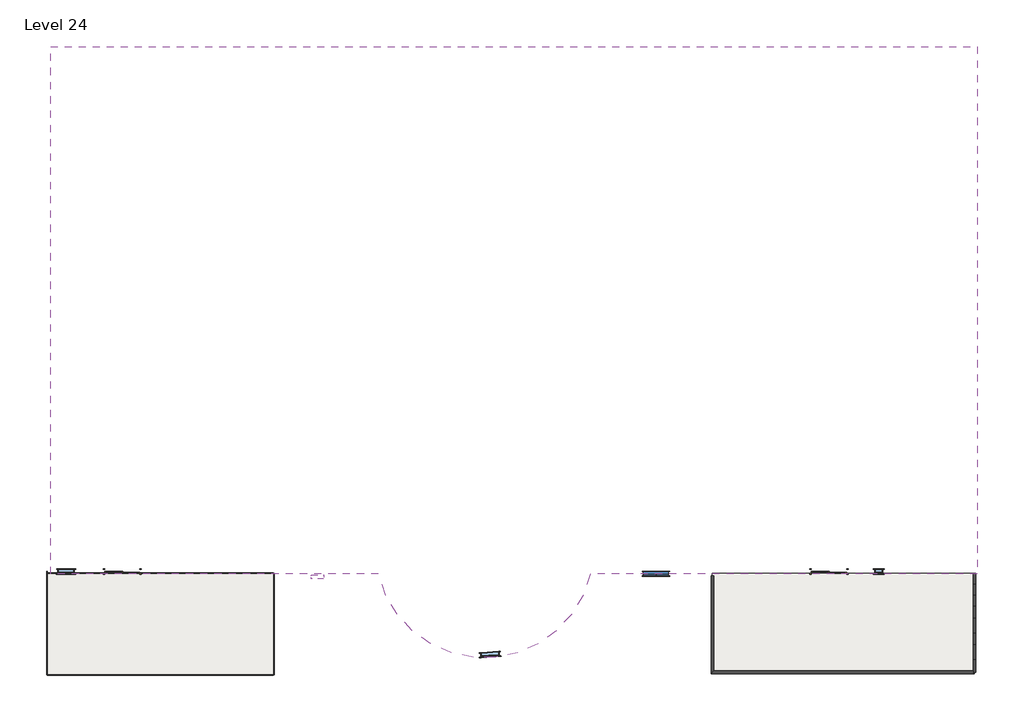
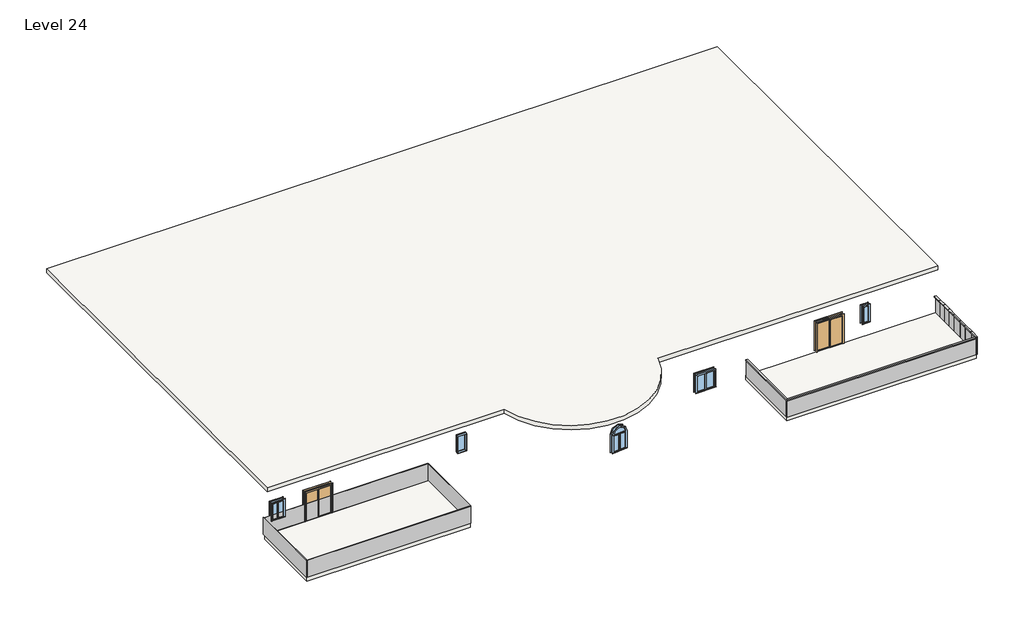
# One storey: 14 plates, 11 members, 5 windows, 3 slabs, 2 doors.
"""IFC4 building model written with IfcOpenShell, lengths in millimetres."""

from ifc_helpers import new_model, si_unit, point, frame, frame_2d, origin, place, context, project, spatial, polyline, circle_curve, trimmed, segment, composite_curve, outline, extrude, transform, mapped, element, save
from components import door_076b30e0, member_75074519, member_47bfaf8a, member_ae70dd35, member_41daa855, member_b9da2caa, member_623bfa76, member_d7af48b5, member_0d72fb60, system_panel_glazed_7af1c9c3, system_panel_glazed_a854efd3, system_panel_glazed_e5e35a93, system_panel_glazed_70ce58d2, system_panel_glazed_b1e6bfa8, system_panel_glazed_da164243, system_panel_glazed_d9f0472a, system_panel_glazed_b96adab1, system_panel_glazed_773201f3, system_panel_glazed_8ecd3908, window_cf4adaea, window_a765b88f, window_bb17773d, window_0862ab64, window_80bd9af0

model = new_model("IFC4")

# Units and contexts
model_context = context("Model", 3, world=origin())
ifc_project = project(units=[si_unit("LENGTHUNIT", "METRE", prefix="MILLI")], contexts=[model_context])

# Site, building, storey
site = spatial("IfcSite", under=ifc_project)
building = spatial("IfcBuilding", under=site)
storey = spatial("IfcBuildingStorey", under=building, Name="Level 24", Elevation=39928.8)

# Doors
placement = place(None, origin())
door_shape = door_076b30e0(model_context)
element("IfcDoor", 1, ObjectType="Door-Double-Sliding : 68\" x 80\"", at=placement, inside=storey, context=model_context, shape_type="MappedRepresentation", body=[
    mapped(door_shape, transform((-16166.185279, -12227.7237084, 39928.8), x_axis=(-1.0, 0.0, 0.0), y_axis=(0.0, -1.0, 0.0), z_axis=(0.0, 0.0, 1.0))),
])
element("IfcDoor", 2, ObjectType="Door-Double-Sliding : 68\" x 80\"", at=placement, inside=storey, context=model_context, shape_type="MappedRepresentation", body=[
    mapped(door_shape, transform((18377.814721, -12227.7237084, 39928.8), x_axis=(-1.0, 0.0, 0.0), y_axis=(0.0, -1.0, 0.0), z_axis=(0.0, 0.0, 1.0))),
])

# Members
member_shape = member_75074519(model_context)
element("IfcMember", 3, ObjectType="Rectangular Mullion : 2.5\" x 5\" rectangular", at=placement, inside=storey, context=model_context, shape_type="MappedRepresentation", body=[
    mapped(member_shape, transform((25489.814721, -17286.7294032, 41148.0), x_axis=(1.0, 0.0, 0.0), y_axis=(0.0, 1.0, 0.0), z_axis=(0.0, 0.0, 1.0))),
])
member_2_shape = member_47bfaf8a(model_context)
element("IfcMember", 4, ObjectType="Rectangular Mullion : 2.5\" x 5\" rectangular", at=placement, inside=storey, context=model_context, shape_type="MappedRepresentation", body=[
    mapped(member_2_shape, transform((25489.814721, -14645.1294032, 41148.0), x_axis=(0.0, 0.0, 1.0), y_axis=(-1.0, 0.0, 0.0), z_axis=(0.0, -1.0, 0.0))),
])
member_3_shape = member_ae70dd35(model_context)
element("IfcMember", 5, ObjectType="Rectangular Mullion : 2.5\" x 5\" rectangular", at=placement, inside=storey, context=model_context, shape_type="MappedRepresentation", body=[
    mapped(member_3_shape, transform((25489.814721, -15356.3294032, 41148.0), x_axis=(0.0, 0.0, 1.0), y_axis=(-1.0, 0.0, 0.0), z_axis=(0.0, -1.0, 0.0))),
])
element("IfcMember", 6, ObjectType="Rectangular Mullion : 2.5\" x 5\" rectangular", at=placement, inside=storey, context=model_context, shape_type="MappedRepresentation", body=[
    mapped(member_2_shape, transform((25489.814721, -17286.7294032, 41148.0), x_axis=(0.0, 0.0, 1.0), y_axis=(-1.0, 0.0, 0.0), z_axis=(0.0, -1.0, 0.0))),
])
member_4_shape = member_41daa855(model_context)
element("IfcMember", 7, ObjectType="Rectangular Mullion : 2.5\" x 5\" rectangular", at=placement, inside=storey, context=model_context, shape_type="MappedRepresentation", body=[
    mapped(member_4_shape, transform((12687.3363499, -12564.9789867, 41148.0), x_axis=(0.0, 0.0, 1.0), y_axis=(1.0, 0.0, 0.0), z_axis=(0.0, 1.0, 0.0))),
])
member_5_shape = member_b9da2caa(model_context)
element("IfcMember", 8, ObjectType="Rectangular Mullion : 2.5\" x 5\" rectangular", at=placement, inside=storey, context=model_context, shape_type="MappedRepresentation", body=[
    mapped(member_5_shape, transform((25489.814721, -12982.7256066, 41148.0), x_axis=(0.0, 0.0, 1.0), y_axis=(-1.0, 0.0, 0.0), z_axis=(0.0, -1.0, 0.0))),
])
element("IfcMember", 9, ObjectType="Rectangular Mullion : 2.5\" x 5\" rectangular", at=placement, inside=storey, context=model_context, shape_type="MappedRepresentation", body=[
    mapped(member_5_shape, transform((25489.814721, -13509.1275049, 41148.0), x_axis=(0.0, 0.0, 1.0), y_axis=(-1.0, 0.0, 0.0), z_axis=(0.0, -1.0, 0.0))),
])
element("IfcMember", 10, ObjectType="Rectangular Mullion : 2.5\" x 5\" rectangular", at=placement, inside=storey, context=model_context, shape_type="MappedRepresentation", body=[
    mapped(member_5_shape, transform((25489.814721, -14035.5294032, 41148.0), x_axis=(0.0, 0.0, 1.0), y_axis=(-1.0, 0.0, 0.0), z_axis=(0.0, -1.0, 0.0))),
])
member_6_shape = member_623bfa76(model_context)
element("IfcMember", 11, ObjectType="Rectangular Mullion : 2.5\" x 5\" rectangular", at=placement, inside=storey, context=model_context, shape_type="MappedRepresentation", body=[
    mapped(member_6_shape, transform((25489.814721, -15940.5294032, 41148.0), x_axis=(0.0, 0.0, 1.0), y_axis=(-1.0, 0.0, 0.0), z_axis=(0.0, -1.0, 0.0))),
])
member_7_shape = member_d7af48b5(model_context)
element("IfcMember", 12, ObjectType="Rectangular Mullion : 2.5\" x 5\" rectangular", at=placement, inside=storey, context=model_context, shape_type="MappedRepresentation", body=[
    mapped(member_7_shape, transform((25489.814721, -16677.1294032, 41148.0), x_axis=(0.0, 0.0, 1.0), y_axis=(-1.0, 0.0, 0.0), z_axis=(0.0, -1.0, 0.0))),
])
member_8_shape = member_0d72fb60(model_context)
element("IfcMember", 13, ObjectType="Rectangular Mullion : 2.5\" x 5\" rectangular", at=placement, inside=storey, context=model_context, shape_type="MappedRepresentation", body=[
    mapped(member_8_shape, transform((12687.3363499, -17286.7294032, 41148.0), x_axis=(0.0, 0.0, 1.0), y_axis=(0.0, 1.0, 0.0), z_axis=(-1.0, 0.0, 0.0))),
])

# Plates
system_panel_glazed_shape = system_panel_glazed_7af1c9c3(model_context)
element("IfcPlate", 14, ObjectType="System Panel : Glazed", at=placement, inside=storey, context=model_context, shape_type="MappedRepresentation", body=[
    mapped(system_panel_glazed_shape, transform((25489.814721, -16981.9294032, 39928.8), x_axis=(0.0, -1.0, 0.0), y_axis=(1.0, 0.0, 0.0), z_axis=(0.0, 0.0, 1.0))),
])
element("IfcPlate", 15, ObjectType="System Panel : Glazed", at=placement, inside=storey, context=model_context, shape_type="MappedRepresentation", body=[
    mapped(system_panel_glazed_shape, transform((25489.814721, -14340.3294032, 39928.8), x_axis=(0.0, -1.0, 0.0), y_axis=(1.0, 0.0, 0.0), z_axis=(0.0, 0.0, 1.0))),
])
system_panel_glazed_2_shape = system_panel_glazed_a854efd3(model_context)
element("IfcPlate", 16, ObjectType="System Panel : Glazed", at=placement, inside=storey, context=model_context, shape_type="MappedRepresentation", body=[
    mapped(system_panel_glazed_2_shape, transform((25489.814721, -15000.7294032, 39928.8), x_axis=(0.0, -1.0, 0.0), y_axis=(1.0, 0.0, 0.0), z_axis=(0.0, 0.0, 1.0))),
])
system_panel_glazed_3_shape = system_panel_glazed_e5e35a93(model_context)
element("IfcPlate", 17, ObjectType="System Panel : Glazed", at=placement, inside=storey, context=model_context, shape_type="MappedRepresentation", body=[
    mapped(system_panel_glazed_3_shape, transform((12687.3363499, -14925.8541949, 39928.8), x_axis=(0.0, 1.0, 0.0), y_axis=(-1.0, 0.0, 0.0), z_axis=(0.0, 0.0, 1.0))),
])
system_panel_glazed_4_shape = system_panel_glazed_70ce58d2(model_context)
element("IfcPlate", 18, ObjectType="System Panel : Glazed", at=placement, inside=storey, context=model_context, shape_type="MappedRepresentation", body=[
    mapped(system_panel_glazed_4_shape, transform((25489.814721, -12719.5246575, 39928.8), x_axis=(0.0, -1.0, 0.0), y_axis=(1.0, 0.0, 0.0), z_axis=(0.0, 0.0, 1.0))),
])
element("IfcPlate", 19, ObjectType="System Panel : Glazed", at=placement, inside=storey, context=model_context, shape_type="MappedRepresentation", body=[
    mapped(system_panel_glazed_4_shape, transform((25489.814721, -13772.3284541, 39928.8), x_axis=(0.0, -1.0, 0.0), y_axis=(1.0, 0.0, 0.0), z_axis=(0.0, 0.0, 1.0))),
])
element("IfcPlate", 20, ObjectType="System Panel : Glazed", at=placement, inside=storey, context=model_context, shape_type="MappedRepresentation", body=[
    mapped(system_panel_glazed_4_shape, transform((25489.814721, -13245.9265558, 39928.8), x_axis=(0.0, -1.0, 0.0), y_axis=(1.0, 0.0, 0.0), z_axis=(0.0, 0.0, 1.0))),
])
system_panel_glazed_5_shape = system_panel_glazed_b1e6bfa8(model_context)
element("IfcPlate", 21, ObjectType="System Panel : Glazed", at=placement, inside=storey, context=model_context, shape_type="MappedRepresentation", body=[
    mapped(system_panel_glazed_5_shape, transform((25489.814721, -16308.8294032, 39928.8), x_axis=(0.0, -1.0, 0.0), y_axis=(1.0, 0.0, 0.0), z_axis=(0.0, 0.0, 1.0))),
])
system_panel_glazed_6_shape = system_panel_glazed_da164243(model_context)
element("IfcPlate", 22, ObjectType="System Panel : Glazed", at=placement, inside=storey, context=model_context, shape_type="MappedRepresentation", body=[
    mapped(system_panel_glazed_6_shape, transform((25489.814721, -15648.4294032, 39928.8), x_axis=(0.0, -1.0, 0.0), y_axis=(1.0, 0.0, 0.0), z_axis=(0.0, 0.0, 1.0))),
])
system_panel_glazed_7_shape = system_panel_glazed_d9f0472a(model_context)
element("IfcPlate", 23, ObjectType="System Panel : Glazed", at=placement, inside=storey, context=model_context, shape_type="MappedRepresentation", body=[
    mapped(system_panel_glazed_7_shape, transform((19056.8255355, -17286.7294032, 39928.8), x_axis=(-1.0, 0.0, 0.0), y_axis=(0.0, -1.0, 0.0), z_axis=(0.0, 0.0, 1.0))),
])
system_panel_glazed_8_shape = system_panel_glazed_b96adab1(model_context)
element("IfcPlate", 24, ObjectType="System Panel : Glazed", at=placement, inside=storey, context=model_context, shape_type="MappedRepresentation", body=[
    mapped(system_panel_glazed_8_shape, transform((-14302.7926538, -12456.3237084, 39928.8), x_axis=(1.0, 0.0, 0.0), y_axis=(0.0, 1.0, 0.0), z_axis=(0.0, 0.0, 1.0))),
])
element("IfcPlate", 25, ObjectType="System Panel : Glazed", at=placement, inside=storey, context=model_context, shape_type="MappedRepresentation", body=[
    mapped(system_panel_glazed_8_shape, transform((-14302.7926538, -17395.7250056, 39928.8), x_axis=(-1.0, 0.0, 0.0), y_axis=(0.0, -1.0, 0.0), z_axis=(0.0, 0.0, 1.0))),
])
system_panel_glazed_9_shape = system_panel_glazed_773201f3(model_context)
element("IfcPlate", 26, ObjectType="System Panel : Glazed", at=placement, inside=storey, context=model_context, shape_type="MappedRepresentation", body=[
    mapped(system_panel_glazed_9_shape, transform((-8781.8000285, -14926.024357, 39928.8), x_axis=(0.0, -1.0, 0.0), y_axis=(1.0, 0.0, 0.0), z_axis=(0.0, 0.0, 1.0))),
])
system_panel_glazed_10_shape = system_panel_glazed_8ecd3908(model_context)
element("IfcPlate", 27, ObjectType="System Panel : Glazed", at=placement, inside=storey, context=model_context, shape_type="MappedRepresentation", body=[
    mapped(system_panel_glazed_10_shape, transform((-19823.785279, -14875.224357, 39928.8), x_axis=(0.0, 1.0, 0.0), y_axis=(-1.0, 0.0, 0.0), z_axis=(0.0, 0.0, 1.0))),
])

# Slabs
element("IfcSlab", 28, ObjectType="Generic - 12\"", at=placement, inside=storey, context=model_context, shape_type="SweptSolid", body=[
    extrude(outline(composite_curve([segment(polyline([(25642.214721, 13328.8447861), (25642.214721, -12477.5552139), (6723.9594464, -12477.5552139)]), True, "CONTINUOUS"), segment(trimmed(circle_curve(frame_2d((1537.614721, -11246.9221727)), 5330.3498284), [point((6723.9594464, -12477.5552139))], [point((-3648.7300045, -12477.5552139))], False, "CARTESIAN"), True, "CONTINUOUS"), segment(polyline([(-3648.7300045, -12477.5552139), (-19671.385279, -12477.5552139), (-19671.385279, 13328.8447861), (25642.214721, 13328.8447861)]), True, "CONTINUOUS")], self_intersect=False)), frame((0.0, 0.0, 42963.6098476), z_axis=(0.0, 0.0, 1.0), x_axis=(1.0, 0.0, 0.0)), (0.0, 0.0, 1.0), 304.8),
])
element("IfcSlab", 29, ObjectType="Generic - 12\"", at=placement, inside=storey, context=model_context, shape_type="SweptSolid", body=[
    extrude(outline(polyline([(25489.814721, -12433.2368115), (25489.814721, -17267.6794032), (12687.3363499, -17267.6794032), (12687.3363499, -12433.2368115), (25489.814721, -12433.2368115)])), frame((0.0, 0.0, 39624.0), z_axis=(0.0, 0.0, 1.0), x_axis=(1.0, 0.0, 0.0)), (0.0, 0.0, 1.0), 304.8),
])
element("IfcSlab", 30, ObjectType="Generic - 12\"", at=placement, inside=storey, context=model_context, shape_type="SweptSolid", body=[
    extrude(outline(polyline([(-8781.8000285, -12456.3237084), (-8781.8000285, -17395.7250056), (-19823.785279, -17395.7250056), (-19823.785279, -12456.3237084), (-8781.8000285, -12456.3237084)])), frame((0.0, 0.0, 39624.0), z_axis=(0.0, 0.0, 1.0), x_axis=(1.0, 0.0, 0.0)), (0.0, 0.0, 1.0), 304.8),
])

# Windows
window_shape = window_cf4adaea(model_context)
element("IfcWindow", 31, ObjectType="36\" x 48\"", at=placement, inside=storey, context=model_context, shape_type="MappedRepresentation", body=[
    mapped(window_shape, transform((1821.5964068, -16416.4921108, 39928.8), x_axis=(-0.996612399121061, -0.08224187448108751, 0.0), y_axis=(0.08224187448108751, -0.996612399121061, 0.0), z_axis=(0.0, 0.0, 1.0))),
])
window_2_shape = window_a765b88f(model_context)
element("IfcWindow", 32, ObjectType="Awning with Trim : 16\" x 48\"", at=placement, inside=storey, context=model_context, shape_type="MappedRepresentation", body=[
    mapped(window_2_shape, transform((20816.214721, -12354.7237084, 39928.8), x_axis=(-1.0, 0.0, 0.0), y_axis=(0.0, -1.0, 0.0), z_axis=(0.0, 0.0, 1.0))),
])
window_3_shape = window_bb17773d(model_context)
element("IfcWindow", 33, ObjectType="Casement Dbl with Trim : 32\" x 48\"", at=placement, inside=storey, context=model_context, shape_type="MappedRepresentation", body=[
    mapped(window_3_shape, transform((-18909.385279, -12335.6737084, 39853.6293246), x_axis=(-1.0, 0.0, 0.0), y_axis=(0.0, -1.0, 0.0), z_axis=(0.0, 0.0, 1.0))),
])
window_4_shape = window_0862ab64(model_context)
element("IfcWindow", 34, ObjectType="Casement Dbl with Trim : 48\" x 48\"", at=placement, inside=storey, context=model_context, shape_type="MappedRepresentation", body=[
    mapped(window_4_shape, transform((9924.3594464, -12437.2737084, 39022.1053459), x_axis=(-1.0, 0.0, 0.0), y_axis=(0.0, -1.0, 0.0), z_axis=(0.0, 0.0, 1.0))),
])
window_5_shape = window_80bd9af0(model_context)
element("IfcWindow", 35, ObjectType="Fixed : 24\" x 48\"", at=placement, inside=storey, context=model_context, shape_type="MappedRepresentation", body=[
    mapped(window_5_shape, transform((-6577.685279, -12617.2007309, 40463.3711489), x_axis=(1.0, 0.0, 0.0), y_axis=(0.0, 1.0, 0.0), z_axis=(0.0, 0.0, 1.0))),
])

save(model, "model.ifc")

# Revit data of these elements
# Type "Door-Double-Sliding : 68\" x 80\""
#   Type Mark = "10"
#   Construction Type Id = "opn-d45"
#   Assembly Code = "C1020"
#   Analytic Construction = "Wood frame, double glass door "
#   Thickness = 0' - 2"
#   Thermal Resistance (R) = 1.8150 (h·ft²·°F)/BTU
#   Heat Transfer Coefficient (U) = 0.5510 BTU/(h·ft²·°F)
#   Height = 6' - 8"
#   Rail Width = 0' - 2"
#   Stiles = 0' - 2"
#   Trim Projection Ext = 0' - 1"
#   Trim Projection Int = 0' - 1"
#   Trim Width = 0' - 3"
#   Width = 5' - 8"
#   Define Thermal Properties by = 1
#   Glazing = Glass
#   Panel Material = Wood - Birch - Solid Stained Light Low Gloss
#   Trim Material = Paint - Sienna
#   Visual Light Transmittance = 0
#   Solar Heat Gain Coefficient = 0
#   Function = (empty or 0)
#   Wall Closure = (empty or 0)
# Type "Rectangular Mullion : 2.5\" x 5\" rectangular"
#   built-in parameter 1007304 = 0.416667 (stored number, unit not read)
#   built-in parameter 1007301 = 0.104167 (stored number, unit not read)
#   built-in parameter 1007300 = 0.104167 (stored number, unit not read)
# Type "System Panel : Glazed"
#   Construction Type Id = "GSP4R"
#   Analytic Construction = "1/8 in Pilkington single glazing"
#   Visual Light Transmittance = 0.9
#   Solar Heat Gain Coefficient = 0.86
#   Heat Transfer Coefficient (U) = 1.18115 BTU/(h·ft²·°F)
# Type "Generic - 12\""
#   Assembly Code = "B1010"
#   Function = 0
#   Layers, outside or top first: 1' - 0" no material (function 1)
# Type "36\" x 48\""
#   Type Mark = "38"
#   Construction Type Id = "SGL"
#   Assembly Code = "B2020100"
#   Analytic Construction = "Large single-glazed windows"
#   Visual Light Transmittance = 0.9
#   Solar Heat Gain Coefficient = 0.86
#   Heat Transfer Coefficient (U) = 0.979472 BTU/(h·ft²·°F)
#   Height = 4' - 0"
#   Default Sill Height = 3' - 0"
#   Trim Projection - Ext. = 0' - 0 1/2"
#   Trim Projection - Int. = 0' - 0 3/4"
#   Trim Width - Exterior = 0' - 3 1/2"
#   Trim Width - Interior = 0' - 3 1/2"
#   Width = 3' - 0"
#   Window Inset = 0' - 0 3/4"
#   Define Thermal Properties by = 1
#   Glass Pane Material = Glass
#   Sash Material = Sash
#   Trim Exterior Material = Trim
#   Trim Interior Material = Trim
#   Wall Closure = (empty or 0)
# Type "Awning with Trim : 16\" x 48\""
#   Type Mark = "14"
#   Construction Type Id = "GSP4R"
#   Assembly Code = "B2020100"
#   Analytic Construction = "1/8 in Pilkington single glazing"
#   Visual Light Transmittance = 0.9
#   Solar Heat Gain Coefficient = 0.78
#   Heat Transfer Coefficient (U) = 0.6496 BTU/(h·ft²·°F)
#   Height = 4' - 0"
#   Default Sill Height = 3' - 0"
#   Trim Projection - Ext. = 0' - 0 1/2"
#   Trim Projection - Int. = 0' - 0 3/4"
#   Trim Width - Exterior = 0' - 3 1/2"
#   Trim Width - Interior = 0' - 3 1/2"
#   Width = 1' - 4"
#   Window Inset = 0' - 0 3/4"
#   Define Thermal Properties by = 1
#   Glass Pane Material = Glass
#   Sash Material = Sash
#   Trim Exterior Material = Trim
#   Trim Interior Material = Trim
#   Wall Closure = (empty or 0)
# Type "Casement Dbl with Trim : 32\" x 48\""
#   Type Mark = "36"
#   Construction Type Id = "GSP4R"
#   Assembly Code = "B2020100"
#   Analytic Construction = "1/8 in Pilkington single glazing"
#   Visual Light Transmittance = 0.9
#   Solar Heat Gain Coefficient = 0.78
#   Heat Transfer Coefficient (U) = 0.6496 BTU/(h·ft²·°F)
#   Height = 4' - 0"
#   Default Sill Height = 3' - 0"
#   Trim Projection - Ext. = 0' - 0 1/2"
#   Trim Projection - Int. = 0' - 0 3/4"
#   Trim Width - Exterior = 0' - 3 1/2"
#   Trim Width - Interior = 0' - 3 1/2"
#   Width = 2' - 8"
#   Window Inset = 0' - 0 3/4"
#   Define Thermal Properties by = 1
#   Glass Pane Material = Glass
#   Sash Material = Sash
#   Trim Exterior Material = Trim
#   Trim Interior Material = Trim
#   Wall Closure = (empty or 0)
# Type "Casement Dbl with Trim : 48\" x 48\""
#   Type Mark = "34"
#   Construction Type Id = "GSP4R"
#   Assembly Code = "B2020100"
#   Analytic Construction = "1/8 in Pilkington single glazing"
#   Visual Light Transmittance = 0.9
#   Solar Heat Gain Coefficient = 0.78
#   Heat Transfer Coefficient (U) = 0.6496 BTU/(h·ft²·°F)
#   Height = 4' - 0"
#   Default Sill Height = 3' - 0"
#   Trim Projection - Ext. = 0' - 0 1/2"
#   Trim Projection - Int. = 0' - 0 3/4"
#   Trim Width - Exterior = 0' - 3 1/2"
#   Trim Width - Interior = 0' - 3 1/2"
#   Width = 4' - 0"
#   Window Inset = 0' - 0 3/4"
#   Define Thermal Properties by = 1
#   Glass Pane Material = Glass
#   Sash Material = Sash
#   Trim Exterior Material = Trim
#   Trim Interior Material = Trim
#   Wall Closure = (empty or 0)
# Type "Fixed : 24\" x 48\""
#   Type Mark = "2"
#   Construction Type Id = "GSP4R"
#   Assembly Code = "B2020100"
#   Analytic Construction = "1/8 in Pilkington single glazing"
#   Visual Light Transmittance = 0.9
#   Solar Heat Gain Coefficient = 0.78
#   Heat Transfer Coefficient (U) = 0.6496 BTU/(h·ft²·°F)
#   Height = 4' - 0"
#   Default Sill Height = 3' - 0"
#   Width = 2' - 0"
#   Window Inset = 0' - 0 3/4"
#   Define Thermal Properties by = 1
#   Glass Pane Material = Glass
#   Sash Material = Sash
#   Wall Closure = (empty or 0)
# Elements 1, 2 (IfcDoor, "Door-Double-Sliding : 68\" x 80\"")
#   Phase Created = New Construction
#   Materials on its faces: "Paint - Sienna", "Wood - Birch - Solid Stained Light Low Gloss", "Glass"
# Elements 3, 4, 5, 6, 7, 8, 9, 10, 11, 12, 13 (IfcMember, "Rectangular Mullion : 2.5\" x 5\" rectangular")
#   Phase Created = New Construction
#   Materials on its faces: "Aluminum"
# Elements 14, 15, 16, 17, 18, 19, 20, 21, 22, 23, 24, 25, 26, 27 (IfcPlate, "System Panel : Glazed")
#   Phase Created = New Construction
#   Materials on its faces: "Glass"
# Element 28 (IfcSlab, "Generic - 12\"")
#   Height Offset From Level = 10' - 11.4807"
#   Phase Created = New Construction
#   Materials on its faces: "Default Floor"
# Elements 29, 30 (IfcSlab, "Generic - 12\"")
#   Height Offset From Level = 0' - 0"
#   Phase Created = New Construction
#   Materials on its faces: "Default Floor"
# Element 31 (IfcWindow, "36\" x 48\"")
#   Mark = "22"
#   Phase Created = New Construction
#   Materials on its faces: "Sash", "Trim", "Glass"
# Element 32 (IfcWindow, "Awning with Trim : 16\" x 48\"")
#   Mark = "56"
#   Phase Created = New Construction
#   Materials on its faces: "Sash", "Trim", "Glass"
# Element 33 (IfcWindow, "Casement Dbl with Trim : 32\" x 48\"")
#   Mark = "39"
#   Phase Created = New Construction
#   Materials on its faces: "Sash", "Trim", "Glass"
# Element 34 (IfcWindow, "Casement Dbl with Trim : 48\" x 48\"")
#   Mark = "5"
#   Phase Created = New Construction
#   Materials on its faces: "Sash", "Trim", "Glass"
# Element 35 (IfcWindow, "Fixed : 24\" x 48\"")
#   Mark = "73"
#   Phase Created = New Construction
#   Materials on its faces: "Sash", "Glass"
# Materials
#   "Glass": class "Glass", colour RGB 0 128 192, transparency 0.75, Description = "Soda Lime Glass", Cost = 0
#   "Wood - Birch - Solid Stained Light Low Gloss": class "Wood", colour RGB 210 159 95, transparency 0, Cost = 0
#   "Paint - Sienna": colour RGB 118 70 51, transparency 0, Cost = 0
#   "Sash": class "Wood", colour RGB 224 178 126, transparency 0
#   "Trim": class "Wood", colour RGB 224 178 126, transparency 0
#   "Aluminum": class "Metal", colour RGB 247 247 247, transparency 0, Description = "Aluminum 6061", Cost = 0
#   "Default Floor": colour RGB 128 128 128, transparency 0
